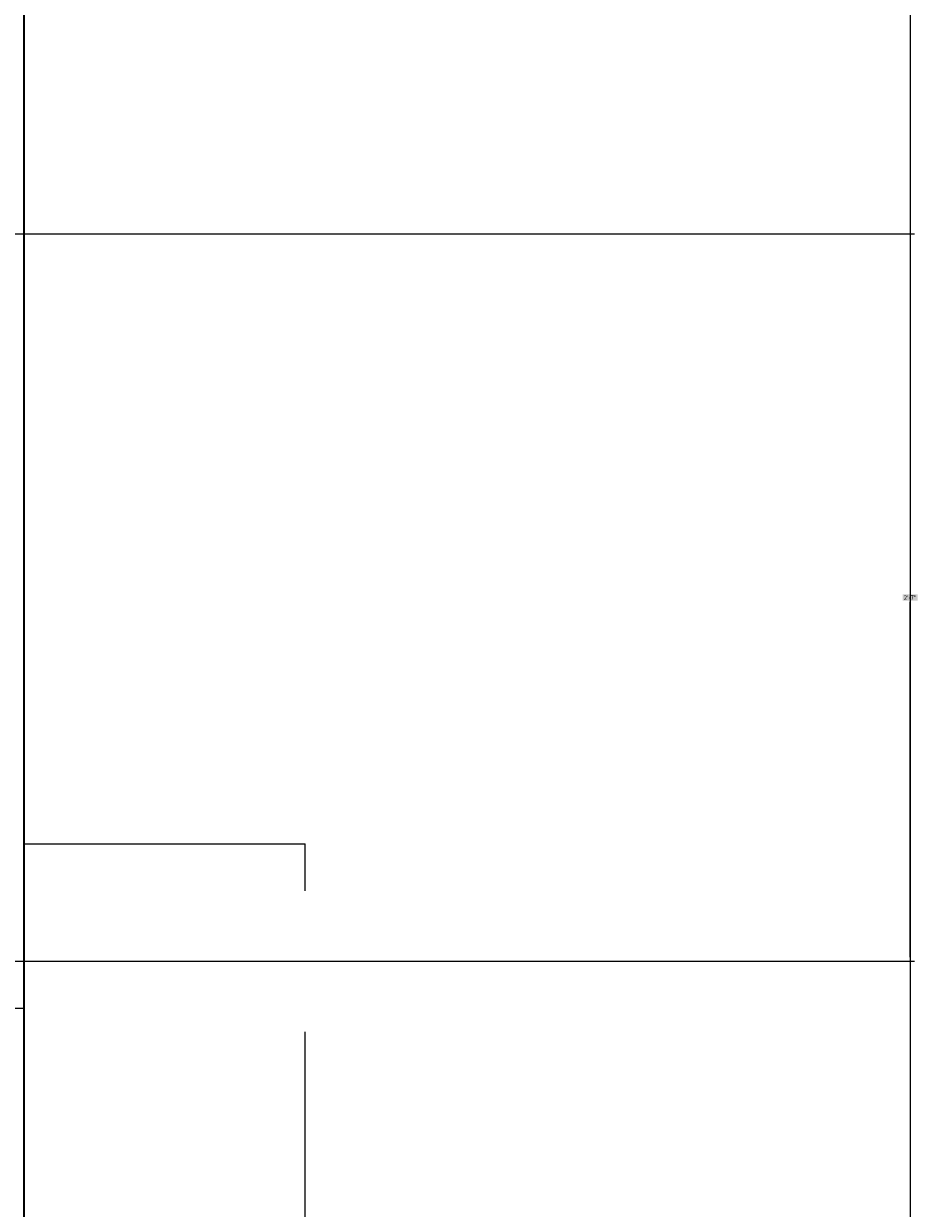
# Model space of a CAD drawing. Units: inches. Extents: x -128 to 854, y -395 to 398.
# Tile 42 of 61: x 314 to 352, y 145 to 196. Entities that reach past the tile are written whole.
import ezdxf

# ---------------------------------------------------------------- set-up
doc = ezdxf.new("R2010")
doc.units = ezdxf.units.IN
doc.header["$MEASUREMENT"] = 0
doc.linetypes.add('ACAD_ISO02W100', pattern=[15, 12, -3])
for name, color, linetype, lineweight in [('A-ANNO-DIMS', 2, 'Continuous', 18), ('A-GLAZ', 220, 'Continuous', 18), ('A-GLAZ-OVHD', 220, 'ACAD_ISO02W100', 13), ('A-WALL', 4, 'Continuous', 35)]:
    doc.layers.add(name, color=color, linetype=linetype, lineweight=lineweight)
doc.styles.get("Standard").update_dxf_attribs({"font": 'arial.ttf'})
doc.dimstyles.get("Standard").update_dxf_attribs({"dimtxt": 0.18, "dimasz": 0.18, "dimexe": 0.18, "dimexo": 0.0625, "dimgap": 0.09, "dimtad": 0, "dimtih": 1, "dimtoh": 1, "dimdec": 1, "dimzin": 0, "dimdsep": 46, "dimlunit": 4, "dimtxsty": 'Standard', "dimcen": 0.09, "dimclrd": 1, "dimclre": 2, "dimclrt": 6, "dimadec": 0, "dimazin": 0, "dimtfac": 1, "dimtdec": 1, "dimtofl": 0, "dimtmove": 0, "dimatfit": 3, "dimfxl": 1, "dimtfill": 2, "dimtfillclr": 3, "dimtolj": 1, "dimtzin": 0, "dimarcsym": 0})

# ---------------------------------------------------------------- blocks, each defined once
blk = doc.blocks.new('WIN-48IN')
for p, q in [((9, 52), (0, 52)), ((9, 50), (0, 50))]:
    blk.add_line(p, q)
blk = doc.blocks.new('SHADE-48IN')
at = {"ltscale": 2}
for p, q in [((12, 62), (0, 62)), ((0, 0), (0, 62)), ((12, 57), (12, 62))]:
    blk.add_line(p, q, dxfattribs=at)
blk = doc.blocks.new('*D98')
at = {"layer": 'A-ANNO-DIMS', "color": 2, "lineweight": -2, "transparency": 16777216}
for p, q in [((313.935, 348.741), (351.853, 348.741)), ((313.935, -89.259), (351.853, -89.259))]:
    blk.add_line(p, q, dxfattribs=at)
at = {"layer": 'A-ANNO-DIMS', "color": 1, "lineweight": -2, "transparency": 16777216}
for p, q in [((351.673, 348.561), (351.673, 129.923)), ((351.673, -89.079), (351.673, 129.559))]:
    blk.add_line(p, q, dxfattribs=at)
at = {"layer": 'A-ANNO-DIMS', "color": 1, "transparency": 16777216}
for points in [[(351.643, 348.561), (351.703, 348.561), (351.673, 348.741)], [(351.643, -89.079), (351.703, -89.079), (351.673, -89.259)]]:
    blk.add_solid(points, dxfattribs=at)
at = {"layer": 'Defpoints', "color": 0, "transparency": 16777216}
for p in [(313.873, 348.741), (351.673, 348.741), (313.873, -89.259)]:
    blk.add_point(p, dxfattribs=at)
at = {"layer": 'A-ANNO-DIMS', "color": 6, "transparency": 16777216, "insert": (351.673, 129.741), "char_height": 0.18, "attachment_point": 5, "bg_fill": 1, "box_fill_scale": 1.25, "bg_fill_color": 3, "bg_fill_transparency": 0}
blk.add_mtext('\\A1;36\'-6"', dxfattribs=at)
blk = doc.blocks.new('*D112')
at = {"layer": 'A-ANNO-DIMS', "color": 2, "lineweight": -2, "transparency": 16777216}
for p, q in [((304.935, 186.741), (351.853, 186.741)), ((304.935, 155.741), (351.853, 155.741))]:
    blk.add_line(p, q, dxfattribs=at)
at = {"layer": 'A-ANNO-DIMS', "color": 1, "lineweight": -2, "transparency": 16777216}
for p, q in [((351.673, 186.561), (351.673, 171.421)), ((351.673, 155.921), (351.673, 171.06))]:
    blk.add_line(p, q, dxfattribs=at)
at = {"layer": 'A-ANNO-DIMS', "color": 1, "transparency": 16777216}
for points in [[(351.643, 186.561), (351.703, 186.561), (351.673, 186.741)], [(351.643, 155.921), (351.703, 155.921), (351.673, 155.741)]]:
    blk.add_solid(points, dxfattribs=at)
at = {"layer": 'Defpoints', "color": 0, "transparency": 16777216}
for p in [(304.873, 186.741), (304.873, 155.741), (351.673, 155.741)]:
    blk.add_point(p, dxfattribs=at)
at = {"layer": 'A-ANNO-DIMS', "color": 6, "transparency": 16777216, "insert": (351.673, 171.241), "char_height": 0.18, "attachment_point": 5, "bg_fill": 1, "box_fill_scale": 1.25, "bg_fill_color": 3, "bg_fill_transparency": 0}
blk.add_mtext('\\A1;2\'-7"', dxfattribs=at)

msp = doc.modelspace()

# ---------------------------------------------------------------- linework, layer by layer
at = {"layer": 'A-WALL'}
msp.add_line((313.873, 348.741), (313.873, -89.259), dxfattribs=at)

# ---------------------------------------------------------------- block references
at = {"layer": 'A-GLAZ', "extrusion": (0, 0, -1), "zscale": -1}
msp.add_blockref('WIN-48IN', (-313.873, 103.741), dxfattribs=at)
at = {"layer": 'A-GLAZ-OVHD', "extrusion": (0, 0, -1), "zscale": -1}
msp.add_blockref('SHADE-48IN', (-325.873, 98.741), dxfattribs=at)

# ---------------------------------------------------------------- dimensions: what is measured, and where the dimension line sits
at = {"layer": 'A-ANNO-DIMS'}
for base, p1, p2, picture, middle in [((351.673, 348.741), (313.873, -89.259), (313.873, 348.741), '*D98', (351.673, 129.741)), ((351.673, 155.741), (304.873, 186.741), (304.873, 155.741), '*D112', (351.673, 171.241))]:
    dim = msp.add_linear_dim(base=base, p1=p1, p2=p2, angle=90, dimstyle='Standard', override={"dimdec": 1, "dimlfac": 1, "dimrnd": 0, "dimzin": 1, "dimdsep": 46, "dimlunit": 4, "dimfrac": 2}, dxfattribs=at)
    dim.commit()
    dim.dimension.update_dxf_attribs({"geometry": picture, "text_midpoint": middle})

doc.saveas('drawing.dxf')
